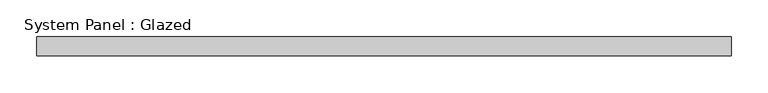
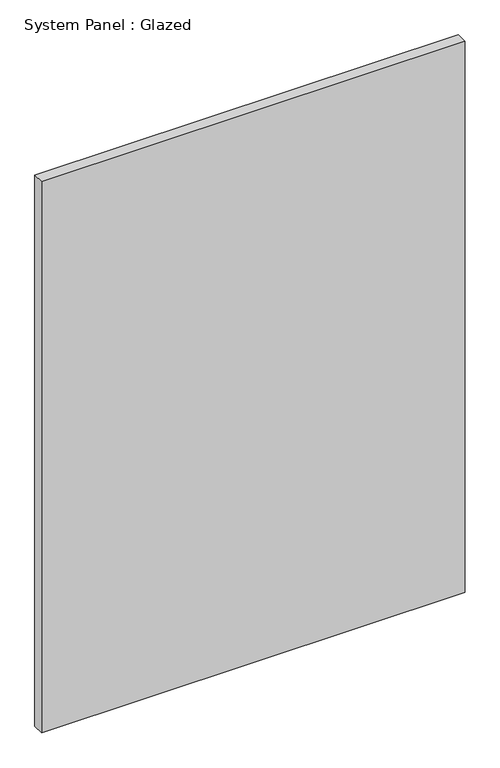
"""IFC4 building model written with IfcOpenShell, lengths in millimetres: plate geometry, System Panel : Glazed."""

from ifc_helpers import new_model, si_unit, origin, origin_with_axes, place, context, project, spatial, polyline, outline, extrude, source, transform, mapped, element, save


def system_panel_glazed_e3ab5e3b(model_context):
    return source(origin(), model_context, "Body", "SweptSolid", [
        extrude(outline(polyline([(469.9, 19.05), (-469.9, 19.05), (-469.9, 44.45), (469.9, 44.45), (469.9, 19.05)])), origin_with_axes(), (0.0, 0.0, 1.0), 1292.092808),
    ])


if __name__ == "__main__":
    model = new_model("IFC4")
    model_context = context("Model", 3, world=origin())
    ifc_project = project(units=[si_unit("LENGTHUNIT", "METRE", prefix="MILLI")], contexts=[model_context])
    site = spatial("IfcSite", under=ifc_project)
    building = spatial("IfcBuilding", under=site)
    placement = place(None, origin())
    system_panel_glazed_shape = system_panel_glazed_e3ab5e3b(model_context)
    element("IfcPlate", 1, ObjectType="System Panel : Glazed", at=placement, inside=building, context=model_context, shape_type="MappedRepresentation", body=[
        mapped(system_panel_glazed_shape, transform((0.0, 0.0, 0.0), x_axis=(1.0, 0.0, 0.0), y_axis=(0.0, 1.0, 0.0), z_axis=(0.0, 0.0, 1.0))),
    ])
    save(model, "model.ifc")

# Revit data of these elements
# Type "System Panel : Glazed"
#   Construction Type Id = "GSP4R"
#   Analytic Construction = "1/8 in Pilkington single glazing"
#   Visual Light Transmittance = 0.9
#   Solar Heat Gain Coefficient = 0.86
#   Heat Transfer Coefficient (U) = 1.18115 BTU/(h·ft²·°F)
#   Define Thermal Properties by = 1
# Element 1 (IfcPlate, "System Panel : Glazed")
#   Materials on its faces: "Glass"
# Materials
#   "Glass": class "Glass", colour RGB 0 128 192, transparency 0.75, Description = "Soda Lime Glass", Cost = 0
